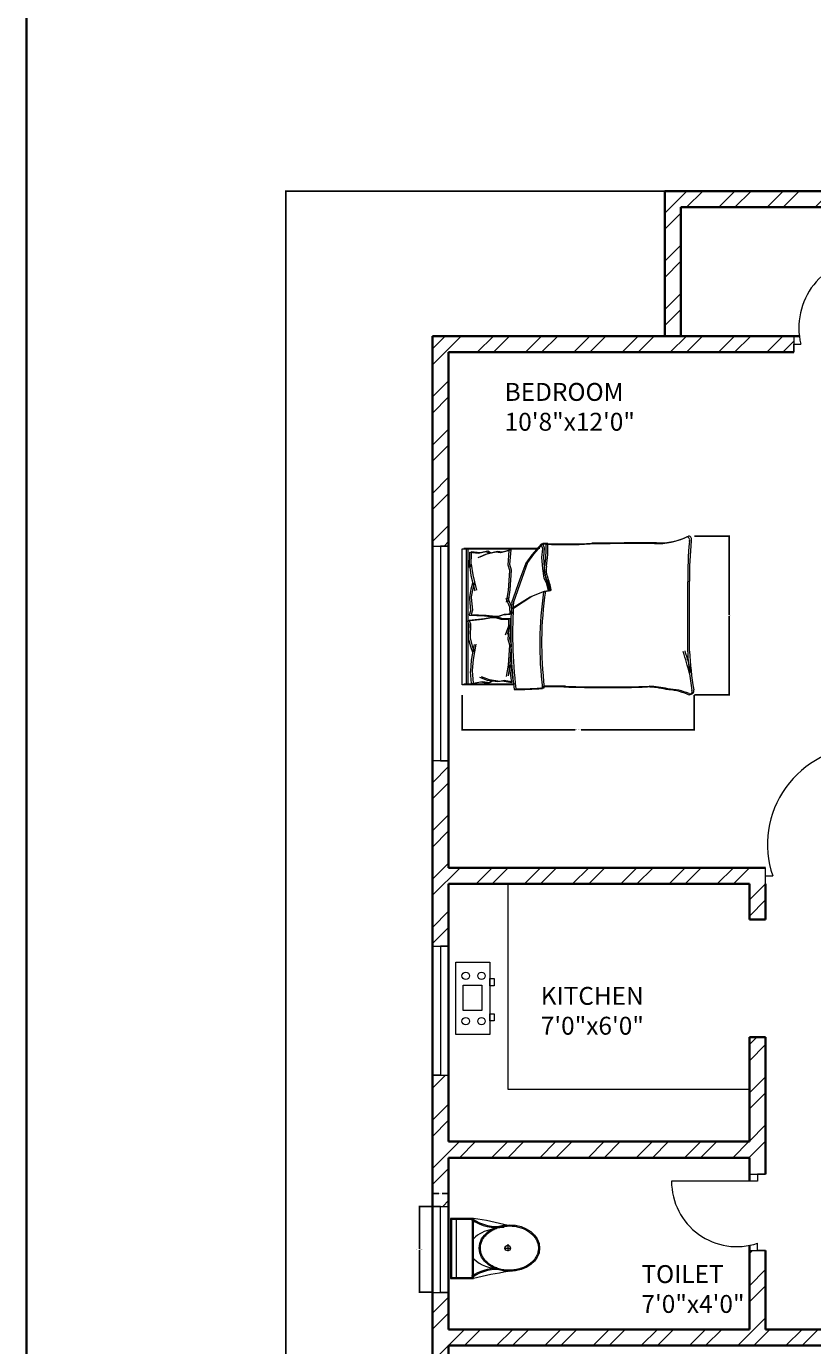
# Model space of a CAD drawing. Units: inches. Extents: x 1944 to 3454, y 1352 to 3055.
# Tile 5 of 17: x 1944 to 2163, y 1900 to 2269. Entities that reach past the tile are written whole.
import ezdxf

# ---------------------------------------------------------------- set-up
doc = ezdxf.new("R2010")
doc.units = ezdxf.units.IN
for name, color, linetype, lineweight in [('A-ANNO-DIMS', 2, 'Continuous', 18), ('A-ANNO-TTLB', 7, 'Continuous', 35), ('A-AREA-IDEN', 7, 'Continuous', 18), ('A-DOOR', 3, 'Continuous', 20), ('A-EQPM', 9, 'Continuous', 18), ('A-FLOR-CASE', 8, 'Continuous', 20), ('A-FLOR-FIXT', 9, 'Continuous', 18), ('A-FURN', 8, 'Continuous', 13), ('A-GLAZ', 4, 'Continuous', 18), ('A-WALL', 7, 'Continuous', 35), ('A-WALL-PATT', 252, 'Continuous', 13)]:
    doc.layers.add(name, color=color, linetype=linetype, lineweight=lineweight)
doc.styles.get("Standard").update_dxf_attribs({"font": 'arial.ttf'})
doc.dimstyles.get("Standard").update_dxf_attribs({"dimtxt": 0.18, "dimasz": 0.18, "dimexe": 0.18, "dimexo": 0.0625, "dimgap": 0.09, "dimtad": 0, "dimtih": 1, "dimtoh": 1, "dimdec": 4, "dimzin": 0, "dimdsep": 46, "dimtxsty": 'Standard', "dimcen": 0.09, "dimadec": 0, "dimazin": 0, "dimtfac": 1, "dimtdec": 4, "dimtofl": 0, "dimtmove": 0, "dimatfit": 3, "dimfxl": 1, "dimtolj": 1, "dimtzin": 0, "dimarcsym": 0})

# ---------------------------------------------------------------- blocks, each defined once
blk = doc.blocks.new('A$C31115884')
for p, q in [((283, 498), (223, 498)), ((258, 466), (258, 523)), ((0, 200), (0, 0)), ((520, 200), (0, 200)), ((10, 190), (10, 10)), ((510, 190), (10, 190)), ((510, 10), (510, 190)), ((520, 0), (520, 200)), ((510, 54), (0, 54)), ((10, 10), (510, 10)), ((0, 0), (520, 0))]:
    blk.add_line(p, q)
blk.add_circle((256, 496), 23.6)
for centre, radius, start, end in [((2778, -205), 2807, 165.4549, 171.7133), ((-295, 403), 365, 324.2091, 9.3499), ((-295, 403), 375, 324.2091, 9.3499), ((806, 403), 365, 170.6501, 215.7909), ((3237, 905), 2807, 188.2867, 194.5451), ((384, 406), 293, 190.2774, 224.1564), ((139, 406), 293, 315.8436, 2.6563), ((806, 403), 375, 179.2036, 215.7909)]:
    blk.add_arc(centre, radius, start, end)
blk.add_ellipse((256, 510), major_axis=(0, -261), ratio=0.772727)
blk.add_open_spline([(256, 259), (263, 259), (270, 260), (288, 262), (299, 265), (320, 273), (330, 278), (350, 291), (360, 299), (378, 316), (386, 326), (402, 347), (409, 358), (421, 383), (427, 395), (436, 422), (440, 436), (445, 465), (447, 480), (448, 509), (448, 524), (445, 553), (443, 568), (436, 596), (432, 610), (422, 636), (416, 649), (402, 672), (395, 683), (379, 703), (370, 712), (351, 728), (341, 735), (321, 746), (310, 751), (289, 757), (278, 759), (256, 761), (245, 761), (223, 757), (212, 754), (191, 746), (181, 741), (161, 728), (151, 720), (133, 703), (125, 693), (110, 672), (103, 660), (90, 636), (85, 623), (76, 596), (72, 582), (67, 553), (66, 538), (64, 509), (65, 494), (68, 465), (70, 450), (77, 422), (81, 408), (91, 382), (97, 370), (111, 346), (118, 335), (135, 316), (144, 307), (162, 291), (172, 284), (193, 273), (203, 269), (225, 262), (236, 260), (250, 259), (253, 259), (256, 259)], degree=3, knots=[0, 0, 0, 0, 0.110105, 0.110105, 0.285049, 0.285049, 0.459994, 0.459994, 0.634938, 0.634938, 0.809882, 0.809882, 0.984827, 0.984827, 1.159771, 1.159771, 1.334715, 1.334715, 1.50966, 1.50966, 1.684604, 1.684604, 1.859549, 1.859549, 2.034493, 2.034493, 2.209437, 2.209437, 2.384382, 2.384382, 2.559326, 2.559326, 2.73427, 2.73427, 2.909215, 2.909215, 3.084159, 3.084159, 3.259103, 3.259103, 3.434048, 3.434048, 3.608992, 3.608992, 3.783936, 3.783936, 3.958881, 3.958881, 4.133825, 4.133825, 4.30877, 4.30877, 4.483714, 4.483714, 4.658658, 4.658658, 4.833603, 4.833603, 5.008547, 5.008547, 5.183491, 5.183491, 5.358436, 5.358436, 5.53338, 5.53338, 5.708324, 5.708324, 5.883269, 5.883269, 6.058213, 6.058213, 6.233158, 6.233158, 6.283185, 6.283185, 6.283185, 6.283185])
blk = doc.blocks.new('BED-WITH-PILLOWS-01')
for p, q in [((0, 40.75), (21.15, 40.75)), ((0, 40.75), (21.15, 40.75)), ((0, 2.76), (0, 40.75)), ((0.51, 40.93), (21.66, 40.93)), ((0.51, 40.93), (21.66, 40.93)), ((1.22, 2.76), (1.22, 40.75)), ((1.22, 2.76), (1.22, 40.75)), ((1.73, 2.94), (1.73, 40.93)), ((1.73, 2.94), (1.73, 40.93)), ((22.05, 42.02), (19.47, 39.08)), ((22.05, 42.02), (19.47, 39.08)), ((22.56, 42.21), (19.98, 39.26)), ((22.56, 42.21), (19.98, 39.26)), ((23.44, 42.09), (22.05, 42.02, 3.08)), ((23.44, 42.09), (22.05, 42.02, 3.08)), ((22.55, 40.8), (22.05, 42.02)), ((22.55, 40.8), (22.05, 42.02)), ((22.3, 38.34), (22.55, 40.8)), ((22.3, 38.34), (22.55, 40.8)), ((23.95, 42.27), (22.56, 42.21, 3.08)), ((23.95, 42.27), (22.56, 42.21, 3.08)), ((23.05, 40.98), (22.56, 42.21)), ((23.05, 40.98), (22.56, 42.21)), ((22.81, 38.52), (23.05, 40.98)), ((22.81, 38.52), (23.05, 40.98)), ((2.03, 39.83), (1.96, 35.54)), ((2.03, 39.83), (1.96, 35.54)), ((2.03, 39.83), (4.58, 39.53)), ((2.03, 39.83), (4.58, 39.53)), ((2.54, 40.01), (2.46, 35.72)), ((2.54, 40.01), (2.46, 35.72)), ((2.54, 40.01), (5.09, 39.71)), ((2.54, 40.01), (5.09, 39.71)), ((6.56, 39.2), (4.43, 38.26)), ((6.56, 39.2), (4.43, 38.26)), ((4.58, 39.53), (6.63, 40.01)), ((4.58, 39.53), (6.63, 40.01)), ((7.07, 39.38), (4.94, 38.44)), ((7.07, 39.38), (4.94, 38.44)), ((5.09, 39.71), (7.14, 40.19)), ((5.09, 39.71), (7.14, 40.19)), ((9.4, 39.83), (6.56, 39.2)), ((9.4, 39.83), (6.56, 39.2)), ((6.63, 40.01), (7.46, 39.6)), ((6.63, 40.01), (7.46, 39.6)), ((9.91, 40.01), (7.07, 39.38)), ((9.91, 40.01), (7.07, 39.38)), ((7.14, 40.19), (7.97, 39.78)), ((7.14, 40.19), (7.97, 39.78)), ((10.68, 39.68), (9.4, 39.83)), ((10.68, 39.68), (9.4, 39.83)), ((11.19, 39.86), (9.91, 40.01)), ((11.19, 39.86), (9.91, 40.01)), ((13.17, 40.3), (10.68, 39.68)), ((13.17, 40.3), (10.68, 39.68)), ((13.68, 40.48), (11.19, 39.86)), ((13.68, 40.48), (11.19, 39.86)), ((12.85, 36.22), (13.17, 40.3)), ((12.85, 36.22), (13.17, 40.3)), ((13.36, 36.4), (13.68, 40.48)), ((13.36, 36.4), (13.68, 40.48)), ((18.26, 36.92), (16.66, 32.49)), ((18.26, 36.92), (16.66, 32.49)), ((19.47, 39.08), (17.75, 36.74)), ((19.47, 39.08), (17.75, 36.74)), ((19.98, 39.26), (18.26, 36.92)), ((19.98, 39.26), (18.26, 36.92)), ((22.55, 35.26), (22.3, 38.34)), ((22.55, 35.26), (22.3, 38.34)), ((23.05, 35.44), (22.81, 38.52)), ((23.05, 35.44), (22.81, 38.52)), ((1.96, 35.54), (2.02, 36.34)), ((1.96, 35.54), (2.02, 36.34)), ((2.02, 36.34), (2.44, 33.32)), ((2.02, 36.34), (2.44, 33.32)), ((2.44, 33.32), (3.51, 29.01)), ((2.44, 33.32), (3.51, 29.01)), ((2.46, 35.72), (2.53, 36.52)), ((2.46, 35.72), (2.53, 36.52)), ((2.53, 36.52), (2.95, 33.5)), ((2.53, 36.52), (2.95, 33.5)), ((2.95, 33.5), (4.02, 29.19)), ((2.95, 33.5), (4.02, 29.19)), ((13.3, 34.66), (12.85, 36.22)), ((13.3, 34.66), (12.85, 36.22)), ((12.95, 29.09), (13.3, 34.66)), ((12.95, 29.09), (13.3, 34.66)), ((13.8, 34.84), (13.36, 36.4)), ((13.8, 34.84), (13.36, 36.4)), ((13.46, 29.27), (13.8, 34.84)), ((13.46, 29.27), (13.8, 34.84)), ((17.75, 36.74), (16.15, 32.31)), ((17.75, 36.74), (16.15, 32.31)), ((22.92, 32.55), (22.55, 35.26)), ((22.92, 32.55), (22.55, 35.26)), ((23.42, 32.74), (23.05, 35.44)), ((23.42, 32.74), (23.05, 35.44)), ((2.45, 29.52), (2.02, 27.19)), ((2.45, 29.52), (2.02, 27.19)), ((2.92, 31.16), (2.45, 29.52)), ((2.92, 31.16), (2.45, 29.52)), ((2.95, 29.7), (2.52, 27.37)), ((2.95, 29.7), (2.52, 27.37)), ((3.43, 31.34), (2.95, 29.7)), ((3.43, 31.34), (2.95, 29.7)), ((16.15, 32.31), (13.82, 25.68)), ((16.15, 32.31), (13.82, 25.68)), ((16.66, 32.49), (14.33, 25.86)), ((16.66, 32.49), (14.33, 25.86)), ((23.65, 30.95), (22.92, 32.55)), ((23.65, 30.95), (22.92, 32.55)), ((24.16, 31.13), (23.42, 32.74)), ((24.16, 31.13), (23.42, 32.74)), ((24.15, 28.98), (23.65, 30.95)), ((24.15, 28.98), (23.65, 30.95)), ((24.65, 29.17), (24.16, 31.13)), ((24.65, 29.16), (24.16, 31.13)), ((62.99, 11.97), (62.99, 31.54)), ((62.99, 11.97), (62.99, 31.54)), ((63.5, 12.16), (63.5, 31.72)), ((63.5, 12.15), (63.5, 31.72)), ((2.02, 27.19), (2.03, 26.93)), ((2.02, 27.19), (2.03, 26.93)), ((2.03, 26.93), (2.37, 23.41)), ((2.03, 26.93), (2.37, 23.41)), ((2.52, 27.37), (2.54, 27.12)), ((2.52, 27.37), (2.54, 27.11)), ((2.54, 27.12), (2.88, 23.6)), ((2.54, 27.11), (2.88, 23.6)), ((13.31, 24.44), (12.28, 26.88)), ((13.31, 24.44), (12.28, 26.88)), ((12.42, 25.88), (12.95, 29.09)), ((12.42, 25.88), (12.95, 29.09)), ((13.81, 24.62), (12.79, 27.07)), ((13.81, 24.62), (12.79, 27.06)), ((12.93, 26.07), (13.46, 29.27)), ((12.93, 26.07), (13.46, 29.27)), ((13.82, 24.05), (18.98, 27.38)), ((13.82, 24.05), (18.98, 27.38)), ((14.33, 24.23), (19.49, 27.56)), ((14.33, 24.23), (19.49, 27.56)), ((18.98, 27.38), (22.55, 28.74)), ((18.98, 27.38), (22.55, 28.74)), ((19.49, 27.56), (23.05, 28.92)), ((19.49, 27.56), (23.05, 28.92)), ((22.55, 28.74), (24.15, 28.98)), ((22.55, 28.74), (24.15, 28.98)), ((23.05, 28.92), (24.65, 29.17)), ((23.05, 28.92), (24.65, 29.16)), ((2.37, 23.41), (1.98, 22.24)), ((2.37, 23.41), (1.98, 22.24)), ((1.98, 22.24), (6.25, 22.04)), ((1.98, 22.24), (6.25, 22.04)), ((2.88, 23.6), (2.49, 22.42)), ((2.88, 23.6), (2.49, 22.42)), ((2.49, 22.42), (6.76, 22.23)), ((2.49, 22.42), (6.76, 22.23)), ((6.76, 22.23), (9.31, 21.93)), ((6.76, 22.23), (9.31, 21.93)), ((9.84, 21.81), (11.3, 22.36)), ((9.84, 21.81), (11.3, 22.36)), ((10.35, 21.99), (11.81, 22.54)), ((10.35, 21.99), (11.81, 22.54)), ((11.3, 22.36), (13.43, 22.49)), ((11.3, 22.36), (13.43, 22.49)), ((11.81, 22.54), (13.94, 22.67)), ((11.81, 22.54), (13.94, 22.67)), ((13.43, 22.49), (13.31, 24.44)), ((13.43, 22.49), (13.31, 24.44)), ((13.94, 22.67), (13.81, 24.62)), ((13.94, 22.67), (13.81, 24.62)), ((1.49, 20.65), (5.74, 21.11)), ((1.49, 20.65), (5.74, 21.11)), ((1.95, 19.5), (1.49, 20.65)), ((1.95, 19.5), (1.49, 20.65)), ((1.83, 15.97), (1.95, 19.5)), ((1.83, 15.97), (1.95, 19.5)), ((1.99, 20.83), (6.25, 21.29)), ((1.99, 20.83), (6.25, 21.29)), ((2.45, 19.69), (1.99, 20.83)), ((2.45, 19.69), (1.99, 20.83)), ((2.34, 16.15), (2.45, 19.69)), ((2.34, 16.15), (2.45, 19.69)), ((5.74, 21.11), (8.27, 21.57)), ((5.74, 21.11), (8.27, 21.57)), ((6.25, 22.04), (8.81, 21.74)), ((6.25, 22.04), (8.81, 21.74)), ((6.25, 21.29), (8.78, 21.75)), ((6.25, 21.29), (8.78, 21.75)), ((8.27, 21.57), (9.3, 21.57)), ((8.27, 21.57), (9.3, 21.57)), ((8.78, 21.75), (9.81, 21.75)), ((8.78, 21.75), (9.81, 21.75)), ((8.81, 21.74), (9.84, 21.81)), ((8.81, 21.74), (9.84, 21.81)), ((9.3, 21.57), (10.8, 21.11)), ((9.3, 21.57), (10.8, 21.11)), ((9.31, 21.93), (10.35, 21.99)), ((9.31, 21.93), (10.35, 21.99)), ((9.81, 21.75), (11.3, 21.29)), ((9.81, 21.75), (11.3, 21.29)), ((10.8, 21.11), (12.93, 21.11)), ((10.8, 21.11), (12.93, 21.11)), ((11.3, 21.29), (13.44, 21.29)), ((11.3, 21.29), (13.44, 21.29)), ((12.93, 19.16), (12.06, 16.66)), ((12.93, 19.16), (12.06, 16.66)), ((13.44, 19.34), (12.57, 16.84)), ((13.44, 19.34), (12.57, 16.84)), ((12.85, 15.41), (13.17, 19.49)), ((12.85, 15.41), (13.17, 19.49)), ((12.93, 21.11), (12.93, 19.16)), ((12.93, 21.11), (12.93, 19.16)), ((13.36, 15.59), (13.68, 19.67)), ((13.36, 15.59), (13.68, 19.67)), ((13.44, 21.29), (13.44, 19.34)), ((13.44, 21.29), (13.44, 19.34)), ((1.83, 15.71), (1.83, 15.97)), ((1.83, 15.71), (1.83, 15.97)), ((2.41, 13.42), (1.83, 15.71)), ((2.41, 13.42), (1.83, 15.71)), ((2.34, 15.9), (2.34, 16.15)), ((2.34, 15.9), (2.34, 16.15)), ((2.91, 13.6), (2.34, 15.9)), ((2.91, 13.6), (2.34, 15.9)), ((13.3, 13.85), (12.85, 15.41)), ((13.3, 13.85), (12.85, 15.41)), ((13.8, 14.03), (13.36, 15.59)), ((13.8, 14.03), (13.36, 15.59)), ((2.98, 11.81), (2.41, 13.42)), ((2.98, 11.81), (2.41, 13.42)), ((2.64, 9.62), (3.44, 13.99)), ((2.64, 9.62), (3.44, 13.99)), ((3.49, 11.99), (2.91, 13.6)), ((3.49, 11.99), (2.91, 13.6)), ((3.14, 9.81), (3.95, 14.17)), ((3.14, 9.81), (3.95, 14.17)), ((12.95, 8.28), (13.3, 13.85)), ((12.95, 8.28), (13.3, 13.85)), ((13.46, 8.46), (13.8, 14.03)), ((13.46, 8.46), (13.8, 14.03)), ((2.41, 6.59), (2.64, 9.62)), ((2.41, 6.59), (2.64, 9.62)), ((2.91, 6.77), (3.14, 9.81)), ((2.91, 6.77), (3.14, 9.81)), ((12.42, 5.07), (12.95, 8.28)), ((12.42, 5.07), (12.95, 8.28)), ((12.93, 5.25), (13.46, 8.46)), ((12.93, 5.25), (13.46, 8.46)), ((12.95, 8.28), (13.21, 7.38)), ((12.95, 8.28), (13.21, 7.38)), ((13.21, 7.38), (13.78, 3.33)), ((13.21, 7.38), (13.78, 3.33)), ((13.46, 8.46), (13.72, 7.56)), ((13.46, 8.46), (13.72, 7.56)), ((13.72, 7.56), (14.29, 3.51)), ((13.72, 7.56), (14.29, 3.51)), ((2.39, 6.5), (2.41, 6.59)), ((2.39, 6.5), (2.41, 6.59)), ((2.65, 3.1), (2.39, 6.5)), ((2.65, 3.1), (2.39, 6.5)), ((2.9, 6.68), (2.91, 6.77)), ((2.9, 6.68), (2.91, 6.77)), ((3.16, 3.28), (2.9, 6.68)), ((3.16, 3.28), (2.9, 6.68)), ((3.14, 3.28), (5.67, 3.74)), ((3.14, 3.28), (5.67, 3.74)), ((7.12, 4.02), (4.93, 4.82)), ((7.12, 4.01), (4.93, 4.82)), ((7.63, 4.2), (5.44, 5)), ((7.63, 4.2), (5.44, 5)), ((5.67, 3.74), (7.74, 3.39)), ((5.67, 3.74), (7.74, 3.39)), ((9.99, 3.56), (7.12, 4.02)), ((9.99, 3.56), (7.12, 4.01)), ((10.5, 3.74), (7.63, 4.2)), ((10.5, 3.74), (7.63, 4.2)), ((7.74, 3.39), (8.55, 3.85)), ((7.74, 3.39), (8.55, 3.85)), ((11.26, 3.79), (9.99, 3.56)), ((11.26, 3.79), (9.99, 3.56)), ((11.76, 3.97), (10.5, 3.74)), ((11.76, 3.97), (10.5, 3.74)), ((13.78, 3.33), (11.26, 3.79)), ((13.78, 3.33), (11.26, 3.79)), ((14.29, 3.51), (11.76, 3.97)), ((14.29, 3.51), (11.76, 3.97)), ((14.4, 2.76), (0, 2.76)), ((14.4, 2.76), (0, 2.76)), ((14.9, 2.94), (0.51, 2.94)), ((14.9, 2.94), (0.51, 2.94)), ((2.64, 3.1), (5.16, 3.56)), ((2.64, 3.1), (5.16, 3.56)), ((5.16, 3.56), (7.23, 3.21)), ((5.16, 3.56), (7.23, 3.21)), ((7.23, 3.21), (8.04, 3.67)), ((7.23, 3.21), (8.04, 3.67))]:
    blk.add_line(p, q)
for centre, radius, start, end in [((55.09, 60.72), 18.33, 267.4714, 296.4681), ((55.09, 60.72), 18.33, 267.4714, 296.4681), ((63.2, 43.43), 0.876, 332.6588, 86.02), ((63.2, 43.43), 0.876, 332.6588, 86.02), ((-5.29, 40.8), 28.76, 349.8763, 2.5657), ((-5.29, 40.8), 28.76, 349.8763, 2.5657), ((28.87, 144.88), 102.94, 266.9791, 273.8365), ((28.87, 144.88), 102.94, 266.9791, 273.8365), ((-4.78, 40.98), 28.76, 349.8763, 2.5657), ((-4.78, 40.98), 28.76, 349.8763, 2.5657), ((29.37, 145.06), 102.94, 266.9791, 273.8365), ((29.37, 145.06), 102.94, 266.9791, 273.8365), ((53.91, -3583.94), 3626.16, 90.00217, 90.28689), ((53.91, -3583.94), 3626.16, 90.00217, 90.28689), ((54.42, -3583.76), 3626.16, 90.00217, 90.28689), ((54.42, -3583.76), 3626.16, 90.00217, 90.28689), ((54.58, 60.54), 18.33, 267.4714, 296.4681), ((54.58, 60.54), 18.33, 267.4714, 296.4681), ((62.69, 43.25), 0.876, 332.6588, 86.02), ((62.69, 43.25), 0.876, 332.6588, 86.02), ((168.74, 32.71), 105.75, 174.4998, 180.6351), ((168.74, 32.71), 105.75, 174.4998, 180.6351), ((169.24, 32.89), 105.75, 174.4998, 180.6351), ((169.24, 32.89), 105.75, 174.4998, 180.6351), ((27.87, 34.77), 4.95, 168.6608, 203.7384), ((27.87, 34.77), 4.95, 168.6608, 203.7384), ((28.38, 34.95), 4.95, 168.6608, 203.7384), ((28.38, 34.95), 4.95, 168.6608, 203.7384), ((1.18, 24.76), 23.57, 10.6617, 19.8806), ((1.18, 24.76), 23.57, 10.6617, 19.8806), ((1.69, 24.95), 23.57, 10.6617, 19.8806), ((1.69, 24.94), 23.57, 10.6617, 19.8806), ((144.71, 16.98), 131.13, 176.0865, 186.7821), ((144.71, 16.98), 131.13, 176.0865, 186.7821), ((145.22, 17.16), 131.13, 176.0865, 186.7821), ((145.22, 17.16), 131.13, 176.0865, 186.7821), ((124.25, 14.11), 102.56, 171.7845, 186.9006), ((124.25, 14.11), 102.56, 171.7845, 186.9006), ((124.76, 14.3), 102.56, 171.7845, 186.9006), ((124.76, 14.3), 102.56, 171.7845, 186.9006), ((24.2, 29.12), 0.147, 250.2464, 1.1377), ((24.2, 29.12), 0.147, 250.2464, 1.1377), ((24.7, 29.3), 0.147, 250.2464, 1.1377), ((24.7, 29.3), 0.147, 250.2464, 1.1377), ((-18.85, -13.69), 84.62, 13.3832, 17.7053), ((-18.85, -13.69), 84.62, 13.3832, 17.7053), ((-18.34, -13.51), 84.62, 13.3832, 17.7053), ((-18.34, -13.51), 84.62, 13.3832, 17.7053), ((159.64, 17.03), 96.78, 182.9958, 189.4091), ((159.64, 17.03), 96.78, 182.9958, 189.4091), ((160.15, 17.21), 96.78, 182.9958, 189.4091), ((160.15, 17.21), 96.78, 182.9958, 189.4091), ((15.97, 67.69), 66.22, 268.7218, 275.604), ((15.97, 67.69), 66.22, 268.7218, 275.604), ((16.48, 67.88), 66.22, 268.7218, 275.604), ((16.48, 67.88), 66.22, 268.7218, 275.604), ((24.78, -132.99), 135.22, 88.4762, 91.0082), ((24.78, -132.99), 135.22, 88.4762, 91.0082), ((25.29, -132.81), 135.22, 88.4762, 91.0082), ((25.29, -132.81), 135.22, 88.4762, 91.0082), ((40.23, 385.38), 383.38, 268.2277, 271.7185), ((40.23, 385.38), 383.38, 268.2277, 271.7185), ((40.74, 385.56), 383.38, 268.2277, 271.7185), ((40.74, 385.56), 383.38, 268.2277, 271.7185), ((51.28, -21.38), 23.56, 76.0648, 88.9113), ((51.28, -21.38), 23.56, 76.0648, 88.9113), ((51.79, -21.2), 23.56, 76.0648, 88.9113), ((51.79, -21.2), 23.56, 76.0648, 88.9113), ((55.86, -17.22), 18.73, 67.9751, 86.652), ((55.86, -17.22), 18.73, 67.9751, 86.652), ((56.37, -17.04), 18.73, 67.9751, 86.652), ((56.37, -17.04), 18.73, 67.9751, 86.652), ((63.37, 0.86), 0.866, 236.1736, 23.4781), ((63.37, 0.86), 0.866, 236.1736, 23.4781), ((63.87, 1.05), 0.866, 236.1736, 23.4781), ((63.87, 1.05), 0.866, 236.1736, 23.4781)]:
    blk.add_arc(centre, radius, start, end)
blk = doc.blocks.new('COOKTOP-4B-01')
for points in [[(0, 20.18), (9.48, 20.18), (9.48, 0), (0, 0)], [(9.48, 15.59), (10.71, 15.59), (10.71, 13.59), (9.48, 13.59)], [(2, 13.79), (7.26, 13.79), (7.26, 6.73), (2, 6.73)], [(9.48, 5.81), (10.71, 5.81), (10.71, 3.8), (9.48, 3.8)]]:
    blk.add_lwpolyline(points, close=True)
for centre in [(2.74, 16.38), (7.14, 16.38), (2.74, 3.71), (7.14, 3.71)]:
    blk.add_circle(centre, 1.05)
blk = doc.blocks.new('DOOR-SWING-36IN-04')
for p, q in [((27.8, 2.25), (27.8, 38.25)), ((0, 0), (0, 4.5)), ((29.8, 4.5), (29.8, 0)), ((0, 2.25), (2, 2.25)), ((29.8, 2.25), (27.8, 2.25)), ((29.8, 0), (29.8, 2.25))]:
    blk.add_line(p, q)
blk.add_arc((27.8, 11), 27.25, 90, 198.7358)
blk = doc.blocks.new('DOOR-SWING-24IN-01')
for p, q in [((20.84, 2.25), (20.84, 26.25)), ((0, 4.5), (0, 0)), ((22.84, 0), (22.84, 4.5)), ((22.84, 4.5), (22.84, 2.25)), ((0, 0), (0, 2.25)), ((0, 2.25), (2, 2.25)), ((22.84, 2.25), (20.84, 2.25))]:
    blk.add_line(p, q)
blk.add_arc((20.84, 6.85), 19.4, 90, 193.7219)
blk = doc.blocks.new('DOOR-SWING-24IN-06')
for p, q in [((24, 19.31), (0, 19.31)), ((21.75, 21.31), (26.25, 21.31)), ((26.25, 21.31), (24, 21.31)), ((24, 21.31), (24, 19.31)), ((24, 0), (24, 2)), ((21.75, 0), (26.25, 0)), ((26.25, 0), (24, 0))]:
    blk.add_line(p, q)
blk.add_arc((18.24, 19.31), 18.24, 180, 288.4122)
blk = doc.blocks.new('WINDOW-PLAN-60.00IN-01')
for p, q in [((0, 60), (4.5, 60)), ((4.5, 60), (2.25, 60)), ((2.25, 60), (2.25, 0)), ((4.5, 0), (0, 0)), ((2.25, 0), (4.5, 0))]:
    blk.add_line(p, q)
blk = doc.blocks.new('WINDOW-PLAN-36.00IN-01')
for p, q in [((0, 36), (4.5, 36)), ((4.5, 36), (2.25, 36)), ((2.25, 36), (2.25, 0)), ((2.25, 0), (0, 0)), ((0, 0), (4.5, 0))]:
    blk.add_line(p, q)
blk = doc.blocks.new('WINDOW-PLAN-24.00IN-01')
for p, q in [((2.25, 24), (0, 24)), ((0, 24), (4.5, 24)), ((2.25, 0), (2.25, 24)), ((0, 0), (4.5, 0)), ((4.5, 0), (2.25, 0))]:
    blk.add_line(p, q)
blk = doc.blocks.new('*D62')
at = {"layer": 'A-ANNO-DIMS', "color": 0, "lineweight": -2, "transparency": 16777216}
for p, q in [((2065.59, 2081.78), (2065.59, 2071.93)), ((2130.41, 2081.78), (2130.41, 2071.93)), ((2065.77, 2072.11), (2097.18, 2072.11)), ((2130.23, 2072.11), (2098.82, 2072.11))]:
    blk.add_line(p, q, dxfattribs=at)
at = {"layer": 'A-ANNO-DIMS', "color": 0, "transparency": 16777216}
for points in [[(2065.77, 2072.14), (2065.77, 2072.08), (2065.59, 2072.11)], [(2130.23, 2072.14), (2130.23, 2072.08), (2130.41, 2072.11)]]:
    blk.add_solid(points, dxfattribs=at)
at = {"layer": 'Defpoints', "color": 0, "transparency": 16777216}
for p in [(2065.59, 2081.84), (2130.41, 2081.84), (2130.41, 2072.11)]:
    blk.add_point(p, dxfattribs=at)
at = {"layer": 'A-ANNO-DIMS', "color": 0, "transparency": 16777216, "insert": (2098, 2072.11), "char_height": 0.18, "attachment_point": 5}
blk.add_mtext('\\A1;BED 65 TYP.', dxfattribs=at)
blk = doc.blocks.new('*D63')
at = {"layer": 'A-ANNO-DIMS', "color": 0, "lineweight": -2, "transparency": 16777216}
for p, q in [((2130.47, 2126.21), (2140.31, 2126.21)), ((2140.13, 2126.03), (2140.13, 2104.21)), ((2140.13, 2082.02), (2140.13, 2103.85)), ((2130.47, 2081.84), (2140.31, 2081.84))]:
    blk.add_line(p, q, dxfattribs=at)
at = {"layer": 'A-ANNO-DIMS', "color": 0, "transparency": 16777216}
for points in [[(2140.1, 2126.03), (2140.16, 2126.03), (2140.13, 2126.21)], [(2140.1, 2082.02), (2140.16, 2082.02), (2140.13, 2081.84)]]:
    blk.add_solid(points, dxfattribs=at)
at = {"layer": 'Defpoints', "color": 0, "transparency": 16777216}
for p in [(2130.41, 2126.21), (2140.13, 2126.21), (2130.41, 2081.84)]:
    blk.add_point(p, dxfattribs=at)
at = {"layer": 'A-ANNO-DIMS', "color": 0, "transparency": 16777216, "insert": (2140.13, 2104.03), "char_height": 0.18, "attachment_point": 5}
blk.add_mtext('\\A1;44 TYP.', dxfattribs=at)
blk = doc.blocks.new('*D74')
at = {"layer": 'A-ANNO-DIMS', "color": 0, "lineweight": -2, "transparency": 16777216}
for p, q in [((2057.26, 1938.98), (2053.54, 1938.98)), ((2053.72, 1938.8), (2053.72, 1927.16)), ((2053.72, 1915.16), (2053.72, 1926.79)), ((2057.26, 1914.98), (2053.54, 1914.98))]:
    blk.add_line(p, q, dxfattribs=at)
at = {"layer": 'A-ANNO-DIMS', "color": 0, "transparency": 16777216}
for points in [[(2053.69, 1938.8), (2053.75, 1938.8), (2053.72, 1938.98)], [(2053.69, 1915.16), (2053.75, 1915.16), (2053.72, 1914.98)]]:
    blk.add_solid(points, dxfattribs=at)
at = {"layer": 'Defpoints', "color": 0, "transparency": 16777216}
for p in [(2053.72, 1938.98), (2057.32, 1938.98), (2057.32, 1914.98)]:
    blk.add_point(p, dxfattribs=at)
at = {"layer": 'A-ANNO-DIMS', "color": 0, "transparency": 16777216, "insert": (2053.72, 1926.98), "char_height": 0.18, "attachment_point": 5}
blk.add_mtext('\\A1;WINDOW 24 TYP.', dxfattribs=at)
blk = doc.blocks.new('*D75')
at = {"layer": 'A-ANNO-DIMS', "color": 0, "lineweight": -2, "transparency": 16777216}
for p, q in [((2057.32, 1939.04), (2057.32, 1942.76)), ((2057.5, 1942.58), (2059.11, 1942.58)), ((2061.64, 1942.58), (2060.03, 1942.58)), ((2061.82, 1939.04), (2061.82, 1942.76))]:
    blk.add_line(p, q, dxfattribs=at)
at = {"layer": 'A-ANNO-DIMS', "color": 0, "transparency": 16777216}
for points in [[(2057.5, 1942.61), (2057.5, 1942.55), (2057.32, 1942.58)], [(2061.64, 1942.61), (2061.64, 1942.55), (2061.82, 1942.58)]]:
    blk.add_solid(points, dxfattribs=at)
at = {"layer": 'Defpoints', "color": 0, "transparency": 16777216}
for p in [(2061.82, 1942.58), (2057.32, 1938.98), (2061.82, 1938.98)]:
    blk.add_point(p, dxfattribs=at)
at = {"layer": 'A-ANNO-DIMS', "color": 0, "transparency": 16777216, "insert": (2059.57, 1942.58), "char_height": 0.18, "attachment_point": 5}
blk.add_mtext('\\A1;5 TYP.', dxfattribs=at)
blk = doc.blocks.new('*D185')
at = {"layer": 'A-ANNO-DIMS', "color": 0, "lineweight": -2, "transparency": 16777216}
for p, q in [((2122.1, 2222.6), (2016.19, 2222.6)), ((2016.37, 2222.42), (2016.37, 1856.28)), ((2016.37, 1489.78), (2016.37, 1855.91)), ((2123.11, 1489.6), (2016.19, 1489.6))]:
    blk.add_line(p, q, dxfattribs=at)
at = {"layer": 'A-ANNO-DIMS', "color": 0, "transparency": 16777216}
for points in [[(2016.34, 2222.42), (2016.4, 2222.42), (2016.37, 2222.6)], [(2016.34, 1489.78), (2016.4, 1489.78), (2016.37, 1489.6)]]:
    blk.add_solid(points, dxfattribs=at)
at = {"layer": 'Defpoints', "color": 0, "transparency": 16777216}
for p in [(2016.37, 2222.6), (2122.17, 2222.6), (2123.17, 1489.6)]:
    blk.add_point(p, dxfattribs=at)
at = {"layer": 'A-ANNO-DIMS', "color": 0, "transparency": 16777216, "insert": (2016.37, 1856.1), "char_height": 0.18, "attachment_point": 5}
blk.add_mtext('\\A1;733', dxfattribs=at)

msp = doc.modelspace()

# ---------------------------------------------------------------- hatches: boundary and pattern name
at = {"layer": 'A-WALL-PATT'}
h = msp.add_hatch(dxfattribs=at)
h.set_pattern_fill('ANSI32', color=256)
h.paths.add_polyline_path([(2061.822, 2177.596), (2158.181, 2177.596), (2158.181, 2179.846), (2158.181, 2182.096), (2057.322, 2182.096), (2057.322, 2123.452), (2061.822, 2123.452)])
h.paths.add_polyline_path([(2258.993, 2179.846), (2258.993, 2182.096), (2218.838, 2182.096), (2218.838, 2177.596), (2258.993, 2177.596)])
h.paths.add_polyline_path([(2315.822, 2177.596), (2322.722, 2177.596), (2322.722, 2182.096), (2303.186, 2182.096), (2303.186, 2177.596), (2311.322, 2177.596), (2311.322, 2033.596), (2231.355, 2033.596), (2231.355, 2029.096), (2311.322, 2029.096), (2311.322, 1904.596), (2307.941, 1904.596), (2307.941, 1900.096), (2319.277, 1900.096), (2319.277, 1902.346), (2319.277, 1904.596), (2315.822, 1904.596), (2315.822, 2029.096), (2394.855, 2029.096), (2394.855, 2033.596), (2315.822, 2033.596)])
h.paths.add_polyline_path([(2407.334, 2182.096), (2366.1, 2182.096), (2366.1, 2177.596), (2407.334, 2177.596), (2407.334, 2179.846)])
h.paths.add_polyline_path([(2440.322, 2177.596), (2443.866, 2177.596), (2443.866, 2182.096), (2431.827, 2182.096), (2431.827, 2179.846), (2431.827, 2177.596), (2435.822, 2177.596), (2435.822, 2033.596), (2430.464, 2033.596), (2430.464, 2029.096), (2445.372, 2029.096), (2445.372, 2031.346), (2445.372, 2033.596), (2440.322, 2033.596)])
h.paths.add_polyline_path([(2569.822, 2182.096), (2466.481, 2182.096), (2466.481, 2177.596), (2565.322, 2177.596), (2565.322, 2123.452), (2569.822, 2123.452)])
h.paths.add_polyline_path([(2569.822, 2063.452), (2567.572, 2063.452), (2565.322, 2063.452), (2565.322, 2033.596), (2478.08, 2033.596), (2476.822, 2033.596), (2476.822, 2028.698), (2476.822, 2020.069), (2481.322, 2020.069), (2481.322, 2029.096), (2565.322, 2029.096), (2565.322, 2014.5), (2569.822, 2014.5)])
h.paths.add_polyline_path([(2569.822, 1978.5), (2565.322, 1978.5), (2565.322, 1957.096), (2481.322, 1957.096), (2481.322, 1990.369), (2476.822, 1990.369), (2476.822, 1957.096), (2476.822, 1952.596), (2476.822, 1947.471), (2481.322, 1947.471), (2481.322, 1952.596), (2565.322, 1952.596), (2565.322, 1943.2), (2569.822, 1943.2)])
h.paths.add_polyline_path([(2569.822, 1919.2), (2565.322, 1919.2), (2565.322, 1904.596), (2481.322, 1904.596), (2481.322, 1928.596), (2476.822, 1928.596), (2476.822, 1904.596), (2350.518, 1904.596), (2350.518, 1900.096), (2476.822, 1900.096), (2565.322, 1900.096), (2565.322, 1895.596), (2565.322, 1887.047), (2569.822, 1887.047)])
h.paths.add_polyline_path([(2280.492, 1904.596), (2150.322, 1904.596), (2150.322, 1926.68), (2148.072, 1926.68), (2145.822, 1926.68), (2145.822, 1904.596), (2061.822, 1904.596), (2061.822, 1914.977), (2059.572, 1914.977), (2057.322, 1914.977), (2057.322, 1887.362), (2061.822, 1887.362), (2061.822, 1900.096), (2150.322, 1900.096), (2280.492, 1900.096), (2280.492, 1902.346)])
h.paths.add_polyline_path([(2150.322, 1957.096), (2150.322, 1986.22), (2145.822, 1986.22), (2145.822, 1957.096), (2061.822, 1957.096), (2061.822, 1975.678), (2057.322, 1975.678), (2057.322, 1938.977), (2061.822, 1938.977), (2061.822, 1952.596), (2145.822, 1952.596), (2145.822, 1947.985), (2150.322, 1947.985), (2150.322, 1952.596)])
h.paths.add_polyline_path([(2061.822, 2063.452), (2057.322, 2063.452), (2057.322, 2011.678), (2061.822, 2011.678), (2061.822, 2029.096), (2145.288, 2029.096), (2145.822, 2029.096), (2145.822, 2019.118), (2150.322, 2019.118), (2150.322, 2029.096), (2150.322, 2033.596), (2147.022, 2033.596), (2061.822, 2033.596)])
h.paths.add_polyline_path([(2061.822, 1835.596), (2133.822, 1835.596), (2133.822, 1794.415), (2138.322, 1794.415), (2138.322, 1835.596), (2231.726, 1835.596), (2231.726, 1840.096), (2061.822, 1840.096), (2061.822, 1851.362), (2057.322, 1851.362), (2057.322, 1810.528), (2061.822, 1810.528)])
h.paths.add_polyline_path([(2061.822, 1774.528), (2059.572, 1774.528), (2057.322, 1774.528), (2057.322, 1723.746), (2061.822, 1723.746), (2061.822, 1735.096), (2133.822, 1735.096), (2133.822, 1731.415), (2138.322, 1731.415), (2138.322, 1759.737), (2133.822, 1759.737), (2133.822, 1739.596), (2061.822, 1739.596)])
h.paths.add_polyline_path([(2061.822, 1678.596), (2147.597, 1678.596), (2147.597, 1680.846), (2147.597, 1683.096), (2138.322, 1683.096), (2138.322, 1710.66), (2136.072, 1710.66), (2133.822, 1710.66), (2133.822, 1683.096), (2061.822, 1683.096), (2061.822, 1699.746), (2057.322, 1699.746), (2057.322, 1645.751), (2061.822, 1645.751)])
h.paths.add_polyline_path([(2061.822, 1585.751), (2057.322, 1585.751), (2057.322, 1530.096), (2158.703, 1530.096), (2158.703, 1534.596), (2061.822, 1534.596)])
h.paths.add_polyline_path([(2191.322, 1678.596), (2195.889, 1678.596), (2195.889, 1683.096), (2181.763, 1683.096), (2181.763, 1680.846), (2181.763, 1678.596), (2186.822, 1678.596), (2186.822, 1534.596), (2181.354, 1534.596), (2181.354, 1530.096), (2196.54, 1530.096), (2196.54, 1532.346), (2196.54, 1534.596), (2191.322, 1534.596)])
h.paths.add_polyline_path([(2315.822, 1678.596), (2402.014, 1678.596), (2402.014, 1683.096), (2355.822, 1683.096), (2355.822, 1835.596), (2360.838, 1835.596), (2360.838, 1840.096), (2351.322, 1840.096), (2351.322, 1683.096), (2273.322, 1683.096), (2273.322, 1840.096), (2263.134, 1840.096), (2263.134, 1837.846), (2263.134, 1835.596), (2268.822, 1835.596), (2268.822, 1683.096), (2227.793, 1683.096), (2227.793, 1678.596), (2311.322, 1678.596), (2311.322, 1534.596), (2302.384, 1534.596), (2302.384, 1530.096), (2324.521, 1530.096), (2324.521, 1532.346), (2324.521, 1534.596), (2315.822, 1534.596)])
h.paths.add_polyline_path([(2440.322, 1678.596), (2443.656, 1678.596), (2443.656, 1683.096), (2432.614, 1683.096), (2432.614, 1680.846), (2432.614, 1678.596), (2435.822, 1678.596), (2435.822, 1534.596), (2440.322, 1534.596)])
h.paths.add_polyline_path([(2409.913, 1534.596), (2369.033, 1534.596), (2369.033, 1530.096), (2409.913, 1530.096)])
h.paths.add_polyline_path([(2259.529, 1532.346), (2259.529, 1534.596), (2218.889, 1534.596), (2218.889, 1532.346), (2218.889, 1530.096), (2259.529, 1530.096)])
h.paths.add_polyline_path([(2569.822, 1584.389), (2567.572, 1584.389), (2565.322, 1584.389), (2565.322, 1534.596), (2465.892, 1534.596), (2465.892, 1530.096), (2569.822, 1530.096)])
h.paths.add_polyline_path([(2505.567, 1530.096), (2501.067, 1530.096), (2501.067, 1494.096), (2381.067, 1494.096), (2381.067, 1530.096), (2376.567, 1530.096), (2376.567, 1489.596), (2381.067, 1489.596), (2505.567, 1489.596), (2505.567, 1494.096)])
h.paths.add_polyline_path([(2127.673, 1530.096), (2123.173, 1530.096), (2123.173, 1489.596), (2127.673, 1489.596), (2252.173, 1489.596), (2252.173, 1494.096), (2252.173, 1530.096), (2247.673, 1530.096), (2247.673, 1494.096), (2127.673, 1494.096)])
h.paths.add_polyline_path([(2251.167, 2222.596), (2126.667, 2222.596), (2122.167, 2222.596), (2122.167, 2182.096), (2126.667, 2182.096), (2126.667, 2218.096), (2210.667, 2218.096), (2234.667, 2218.096), (2246.667, 2218.096), (2246.667, 2182.096), (2251.167, 2182.096), (2251.167, 2218.096)])
h.paths.add_polyline_path([(2501.916, 2222.596), (2497.416, 2222.596), (2372.916, 2222.596), (2372.916, 2218.096), (2372.916, 2182.096), (2377.416, 2182.096), (2377.416, 2218.096), (2497.416, 2218.096), (2497.416, 2182.096), (2501.916, 2182.096)])
h.paths.add_polyline_path([(2569.822, 1700.442), (2565.322, 1700.442), (2565.322, 1683.096), (2493.322, 1683.096), (2493.322, 1709.096), (2488.822, 1709.096), (2488.822, 1683.096), (2475.416, 1683.096), (2475.416, 1680.846), (2475.416, 1678.596), (2488.822, 1678.596), (2565.322, 1678.596), (2565.322, 1644.389), (2569.822, 1644.389)])
h.paths.add_polyline_path([(2569.822, 1773.506), (2565.322, 1773.506), (2565.322, 1739.596), (2493.322, 1739.596), (2493.322, 1754.002), (2488.822, 1754.002), (2488.822, 1729.846), (2491.072, 1729.846), (2493.322, 1729.846), (2493.322, 1735.096), (2565.322, 1735.096), (2565.322, 1724.442), (2569.822, 1724.442)])
h.paths.add_polyline_path([(2569.822, 1851.047), (2567.572, 1851.047), (2565.322, 1851.047), (2565.322, 1840.096), (2395.039, 1840.096), (2395.039, 1837.846), (2395.039, 1835.596), (2488.822, 1835.596), (2488.822, 1798.423), (2493.322, 1798.423), (2493.322, 1835.596), (2565.322, 1835.596), (2565.322, 1809.506), (2569.822, 1809.506)])
h.paths.add_polyline_path([(2347.275, 1955.576), (2414.024, 1955.576), (2414.024, 1974.234), (2347.275, 1974.234)], flags=9)
h.paths.add_polyline_path([(2509.756, 1990.497), (2542.915, 1990.497), (2542.915, 2009.154), (2509.756, 2009.154)], flags=9)

# ---------------------------------------------------------------- linework, layer by layer
at = {"layer": 'A-ANNO-TTLB'}
msp.add_lwpolyline([(1943.914, 3054.605), (3453.633, 3054.605), (3453.633, 1351.76), (1943.914, 1351.76)], close=True, dxfattribs=at)
at = {"layer": 'A-FLOR-CASE'}
for p, q in [((2078.407, 1971.658), (2078.407, 2029.096)), ((2145.822, 1971.658), (2078.407, 1971.658))]:
    msp.add_line(p, q, dxfattribs=at)
at = {"layer": 'A-WALL'}
for p, q in [((2126.667, 2222.596), (2122.167, 2222.596)), ((2122.167, 2222.596), (2122.167, 2182.096)), ((2251.167, 2222.596), (2126.667, 2222.596)), ((2126.667, 2182.096), (2126.667, 2218.096)), ((2126.667, 2218.096), (2210.667, 2218.096)), ((2057.322, 2182.096), (2159.77, 2182.096)), ((2057.322, 2182.096), (2057.322, 1530.096)), ((2061.822, 2177.596), (2158.181, 2177.596)), ((2061.822, 2177.596), (2061.822, 2033.596)), ((2061.822, 2033.596), (2147.022, 2033.596)), ((2150.322, 2033.596), (2147.022, 2033.596)), ((2061.822, 2029.096), (2145.288, 2029.096)), ((2061.822, 2029.096), (2061.822, 1957.096)), ((2145.288, 2029.096), (2145.822, 2029.096)), ((2145.822, 2019.118), (2145.822, 2029.096)), ((2150.322, 2029.096), (2150.322, 2019.118)), ((2145.822, 2019.118), (2150.322, 2019.118)), ((2145.822, 1957.096), (2145.822, 1986.22)), ((2145.822, 1986.22), (2150.322, 1986.22)), ((2150.322, 1986.22), (2150.322, 1957.096)), ((2061.822, 1957.096), (2145.822, 1957.096)), ((2150.322, 1957.096), (2150.322, 1952.596)), ((2145.822, 1952.596), (2061.822, 1952.596)), ((2061.822, 1952.596), (2061.822, 1904.596)), ((2145.822, 1945.985), (2145.822, 1952.596)), ((2150.322, 1952.596), (2150.322, 1947.985)), ((2145.822, 1904.596), (2145.822, 1928.087)), ((2150.322, 1926.68), (2150.322, 1904.596)), ((2061.822, 1904.596), (2145.822, 1904.596)), ((2150.322, 1904.596), (2281.622, 1904.596)), ((2150.322, 1900.096), (2061.822, 1900.096)), ((2061.822, 1900.096), (2061.822, 1840.096)), ((2061.822, 1900.096), (2061.822, 1840.096)), ((2150.322, 1900.096), (2280.492, 1900.096))]:
    msp.add_line(p, q, dxfattribs=at)

# ---------------------------------------------------------------- block references
at = {"layer": 'A-DOOR'}
for name, p in [('DOOR-SWING-24IN-01', (2158.181, 2177.596)), ('DOOR-SWING-36IN-04', (2150.322, 2029.096)), ('DOOR-SWING-24IN-06', (2124.072, 1926.68))]:
    msp.add_blockref(name, p, dxfattribs=at)
at = {"layer": 'A-EQPM'}
msp.add_blockref('COOKTOP-4B-01', (2063.857, 1987.009), dxfattribs=at)
at = {"layer": 'A-FLOR-FIXT', "xscale": 0.0323450304620732, "yscale": 0.0323450304620732, "zscale": 0.0323450304620732, "rotation": 270}
msp.add_blockref('A$C31115884', (2062.305, 1935.624), dxfattribs=at)
at = {"layer": 'A-FURN'}
msp.add_blockref('BED-WITH-PILLOWS-01', (2065.588, 2081.907), dxfattribs=at)
at = {"layer": 'A-GLAZ'}
for name, p in [('WINDOW-PLAN-60.00IN-01', (2057.322, 2063.452)), ('WINDOW-PLAN-36.00IN-01', (2057.322, 1975.678)), ('WINDOW-PLAN-24.00IN-01', (2057.322, 1914.977))]:
    msp.add_blockref(name, p, dxfattribs=at)

# ---------------------------------------------------------------- texts
at = {"layer": 'A-AREA-IDEN', "char_height": 5, "attachment_point": 1}
for s, width, insert in [('BEDROOM\\P10\'8"x12\'0"', 173.11294, (2077.472, 2168.997)), ('KITCHEN\\P7\'0"x6\'0"', 122.07808, (2087.553, 2000.29)), ('TOILET\\P7\'0"x4\'0"', 90.98016, (2115.66, 1922.575))]:
    msp.add_mtext_dynamic_manual_height_columns(s, width=width, gutter_width=12.5, heights=[0], dxfattribs=dict(at, insert=insert))

# ---------------------------------------------------------------- dimensions: what is measured, and where the dimension line sits
at = {"layer": 'A-ANNO-DIMS'}
dim = msp.add_linear_dim(base=(2016.372, 2222.596), p1=(2123.173, 1489.596), p2=(2122.167, 2222.596), angle=90, dimstyle='Standard', override={"dimdec": 0, "dimlfac": 1, "dimrnd": 0, "dimzin": 0, "dimdsep": 46, "dimlunit": 2}, dxfattribs=at)
dim.commit()
dim.dimension.update_dxf_attribs({"geometry": '*D185', "text_midpoint": (2016.372, 1856.096)})
for base, p1, p2, text, picture, middle in [((2140.133, 2126.212), (2130.409, 2081.838), (2130.409, 2126.212), '<> TYP.', '*D63', (2140.133, 2104.025)), ((2053.722, 1938.977), (2057.322, 1914.977), (2057.322, 1938.977), 'WINDOW <> TYP.', '*D74', (2053.722, 1926.977))]:
    dim = msp.add_linear_dim(base=base, p1=p1, p2=p2, angle=90, text=text, dimstyle='Standard', override={"dimdec": 0, "dimlfac": 1, "dimrnd": 0, "dimzin": 0, "dimdsep": 46, "dimlunit": 2}, dxfattribs=at)
    dim.commit()
    dim.dimension.update_dxf_attribs({"geometry": picture, "text_midpoint": middle})
for base, p1, p2, text, picture, middle in [((2130.409, 2072.115), (2065.588, 2081.838), (2130.409, 2081.838), 'BED <> TYP.', '*D62', (2097.998, 2072.115)), ((2061.821802765, 1942.576527537), (2057.321802765, 1938.976527537), (2061.821802765, 1938.976527537), '<> TYP.', '*D75', (2059.571802765, 1942.576527537))]:
    dim = msp.add_linear_dim(base=base, p1=p1, p2=p2, text=text, dimstyle='Standard', override={"dimdec": 0, "dimlfac": 1, "dimrnd": 0, "dimzin": 0, "dimdsep": 46, "dimlunit": 2}, dxfattribs=at)
    dim.commit()
    dim.dimension.update_dxf_attribs({"geometry": picture, "text_midpoint": middle})

doc.saveas('drawing.dxf')
